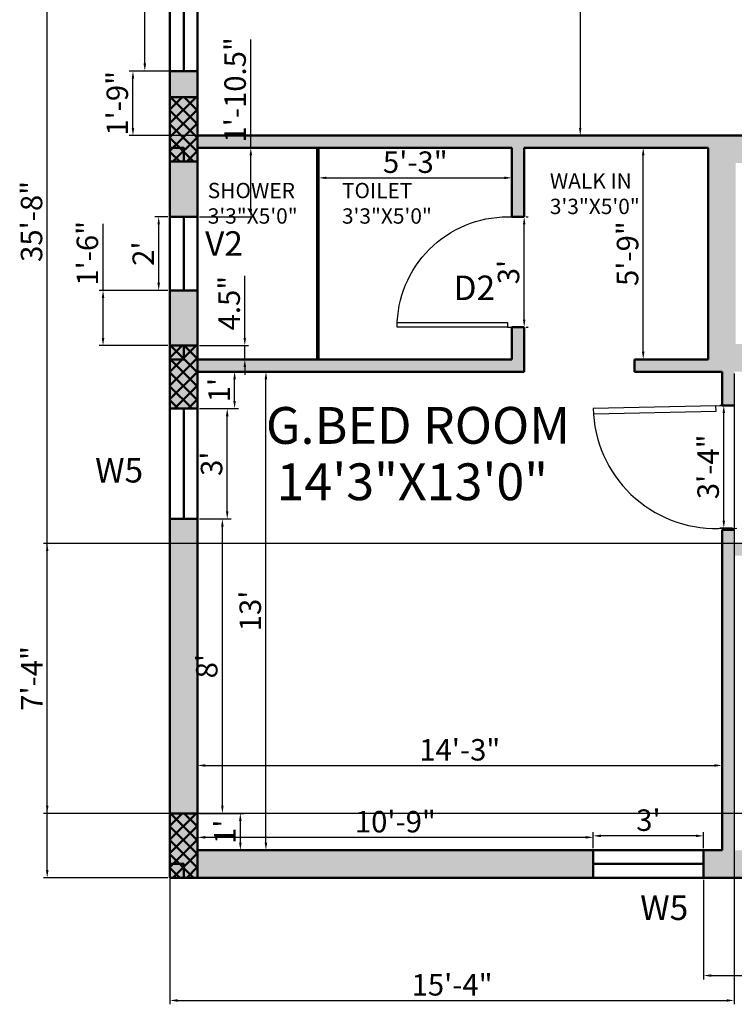
# Model space of a CAD drawing. Units: inches. Extents: x 1749 to 3550, y 1117 to 2383.
# Tile 1 of 15: x 1811 to 2044, y 1169 to 1490. Entities that reach past the tile are written whole.
import ezdxf

# ---------------------------------------------------------------- set-up
doc = ezdxf.new("R2010")
doc.units = ezdxf.units.IN
for name, color, linetype, lineweight in [('A-ANNO-DIMS', 2, 'Continuous', 18), ('A-ANNO-TEXT', 3, 'Continuous', 18), ('A-AREA-IDEN', 7, 'Continuous', 18), ('A-COLS', 10, 'Continuous', 50), ('A-DOOR', 30, 'Continuous', 25), ('A-WALL', 7, 'Continuous', 50), ('A-WALL-PATT', 8, 'Continuous', 13)]:
    doc.layers.add(name, color=color, linetype=linetype, lineweight=lineweight)
doc.styles.get("Standard").update_dxf_attribs({"font": 'arial.ttf'})
doc.dimstyles.new('ISO-25', dxfattribs={"dimtxt": 7, "dimasz": 2.5, "dimexe": 1.25, "dimexo": 0.625, "dimtad": 1, "dimdec": 1, "dimlunit": 3, "dimtxsty": 'Standard', "dimcen": 2.5, "dimadec": 0, "dimazin": 0, "dimtfac": 1, "dimtdec": 1, "dimtmove": 0, "dimatfit": 3, "dimfxl": 1, "dimarcsym": 0})

# ---------------------------------------------------------------- blocks, each defined once
blk = doc.blocks.new('*U12')
for p, q in [((0, 0), (0, 6)), ((40, 0), (40, 6))]:
    blk.add_line(p, q)
blk.add_lwpolyline([(0, 0), (0, -40), (1.75, -40), (1.75, 0)], close=True)
blk.add_arc((0, 0), 40, 270, 0)
blk = doc.blocks.new('*D16')
at = {"layer": 'A-ANNO-DIMS', "color": 0, "lineweight": -2, "ltscale": 0.5, "transparency": 16777216}
for p, q in [((1995.57, 1629.24), (1992.13, 1629.24)), ((1993.38, 1626.74), (1993.38, 1454.74)), ((1995.57, 1452.24), (1992.13, 1452.24))]:
    blk.add_line(p, q, dxfattribs=at)
at = {"layer": 'A-ANNO-DIMS', "color": 0, "ltscale": 0.5, "transparency": 16777216}
for points in [[(1992.96, 1626.74), (1993.8, 1626.74), (1993.38, 1629.24)], [(1992.96, 1454.74), (1993.8, 1454.74), (1993.38, 1452.24)]]:
    blk.add_solid(points, dxfattribs=at)
at = {"layer": 'Defpoints', "color": 0, "ltscale": 0.5, "transparency": 16777216}
for p in [(1996.2, 1629.24), (1993.38, 1452.24), (1996.2, 1452.24)]:
    blk.add_point(p, dxfattribs=at)
at = {"layer": 'A-ANNO-DIMS', "color": 0, "ltscale": 0.5, "transparency": 16777216, "insert": (1989.18, 1540.74), "char_height": 7, "attachment_point": 5, "rotation": 90}
blk.add_mtext('14\'-9"', dxfattribs=at)
blk = doc.blocks.new('*D21')
at = {"layer": 'A-ANNO-DIMS', "color": 0, "lineweight": -2, "ltscale": 0.5, "transparency": 16777216}
for p, q in [((2011.73, 1448.24), (2015.16, 1448.24)), ((2013.91, 1381.74), (2013.91, 1445.74)), ((2011.73, 1379.24), (2015.16, 1379.24))]:
    blk.add_line(p, q, dxfattribs=at)
at = {"layer": 'A-ANNO-DIMS', "color": 0, "ltscale": 0.5, "transparency": 16777216}
for points in [[(2013.49, 1445.74), (2014.33, 1445.74), (2013.91, 1448.24)], [(2013.49, 1381.74), (2014.33, 1381.74), (2013.91, 1379.24)]]:
    blk.add_solid(points, dxfattribs=at)
at = {"layer": 'Defpoints', "color": 0, "ltscale": 0.5, "transparency": 16777216}
for p in [(2011.1, 1448.24), (2013.91, 1448.24), (2011.1, 1379.24)]:
    blk.add_point(p, dxfattribs=at)
at = {"layer": 'A-ANNO-DIMS', "color": 0, "ltscale": 0.5, "transparency": 16777216, "insert": (2009.71, 1413.74), "char_height": 7, "attachment_point": 5, "rotation": 90}
blk.add_mtext('5\'-9"', dxfattribs=at)
blk = doc.blocks.new('*D22')
at = {"layer": 'A-ANNO-DIMS', "color": 0, "lineweight": -2, "ltscale": 0.5, "transparency": 16777216}
for p, q in [((1908.1, 1447.62), (1908.1, 1437.19)), ((1971.1, 1447.62), (1971.1, 1437.19)), ((1910.6, 1438.44), (1968.6, 1438.44))]:
    blk.add_line(p, q, dxfattribs=at)
at = {"layer": 'A-ANNO-DIMS', "color": 0, "ltscale": 0.5, "transparency": 16777216}
for points in [[(1910.6, 1438.86), (1910.6, 1438.03), (1908.1, 1438.44)], [(1968.6, 1438.86), (1968.6, 1438.03), (1971.1, 1438.44)]]:
    blk.add_solid(points, dxfattribs=at)
at = {"layer": 'Defpoints', "color": 0, "ltscale": 0.5, "transparency": 16777216}
for p in [(1908.1, 1448.24), (1971.1, 1448.24), (1971.1, 1438.44)]:
    blk.add_point(p, dxfattribs=at)
at = {"layer": 'A-ANNO-DIMS', "color": 0, "ltscale": 0.5, "transparency": 16777216, "insert": (1939.6, 1442.65), "char_height": 7, "attachment_point": 5}
blk.add_mtext('5\'-3"', dxfattribs=at)
blk = doc.blocks.new('*D23')
at = {"layer": 'A-ANNO-DIMS', "color": 0, "lineweight": -2, "ltscale": 0.5, "transparency": 16777216}
for p, q in [((1869.23, 1375.24), (1892.16, 1375.24)), ((1890.91, 1221.74), (1890.91, 1372.74)), ((1869.23, 1219.24), (1892.16, 1219.24))]:
    blk.add_line(p, q, dxfattribs=at)
at = {"layer": 'A-ANNO-DIMS', "color": 0, "ltscale": 0.5, "transparency": 16777216}
for points in [[(1890.49, 1372.74), (1891.33, 1372.74), (1890.91, 1375.24)], [(1890.49, 1221.74), (1891.33, 1221.74), (1890.91, 1219.24)]]:
    blk.add_solid(points, dxfattribs=at)
at = {"layer": 'Defpoints', "color": 0, "ltscale": 0.5, "transparency": 16777216}
for p in [(1868.6, 1375.24), (1890.91, 1375.24), (1868.6, 1219.24)]:
    blk.add_point(p, dxfattribs=at)
at = {"layer": 'A-ANNO-DIMS', "color": 0, "ltscale": 0.5, "transparency": 16777216, "insert": (1886.71, 1297.24), "char_height": 7, "attachment_point": 5, "rotation": 90}
blk.add_mtext("13'", dxfattribs=at)
blk = doc.blocks.new('*D24')
at = {"layer": 'A-ANNO-DIMS', "color": 0, "lineweight": -2, "ltscale": 0.5, "transparency": 16777216}
for p, q in [((1868.6, 1219.87), (1868.6, 1248.11)), ((1871.1, 1246.86), (2037.1, 1246.86)), ((2039.6, 1219.87), (2039.6, 1248.11))]:
    blk.add_line(p, q, dxfattribs=at)
at = {"layer": 'A-ANNO-DIMS', "color": 0, "ltscale": 0.5, "transparency": 16777216}
for points in [[(1871.1, 1247.28), (1871.1, 1246.44), (1868.6, 1246.86)], [(2037.1, 1247.28), (2037.1, 1246.44), (2039.6, 1246.86)]]:
    blk.add_solid(points, dxfattribs=at)
at = {"layer": 'Defpoints', "color": 0, "ltscale": 0.5, "transparency": 16777216}
for p in [(2039.6, 1246.86), (1868.6, 1219.24), (2039.6, 1219.24)]:
    blk.add_point(p, dxfattribs=at)
at = {"layer": 'A-ANNO-DIMS', "color": 0, "ltscale": 0.5, "transparency": 16777216, "insert": (1954.1, 1251.06), "char_height": 7, "attachment_point": 5}
blk.add_mtext('14\'-3"', dxfattribs=at)
blk = doc.blocks.new('*D61')
at = {"layer": 'A-ANNO-DIMS', "color": 0, "lineweight": -2, "ltscale": 0.5, "transparency": 16777216}
for p, q in [((2033.6, 1209.62), (2033.6, 1177.12)), ((2057.1, 1209.62), (2057.1, 1177.12)), ((2036.1, 1178.37), (2054.6, 1178.37)), ((2057.1, 1178.37), (2092.4, 1178.37))]:
    blk.add_line(p, q, dxfattribs=at)
at = {"layer": 'A-ANNO-DIMS', "color": 0, "ltscale": 0.5, "transparency": 16777216}
for points in [[(2036.1, 1178.79), (2036.1, 1177.95), (2033.6, 1178.37)], [(2054.6, 1178.79), (2054.6, 1177.95), (2057.1, 1178.37)]]:
    blk.add_solid(points, dxfattribs=at)
at = {"layer": 'Defpoints', "color": 0, "ltscale": 0.5, "transparency": 16777216}
for p in [(2033.6, 1210.24), (2057.1, 1210.24), (2057.1, 1178.37)]:
    blk.add_point(p, dxfattribs=at)
at = {"layer": 'A-ANNO-DIMS', "color": 0, "ltscale": 0.5, "transparency": 16777216, "insert": (2076, 1182.57), "char_height": 7, "attachment_point": 5}
blk.add_mtext('1\'-11.5"', dxfattribs=at)
blk = doc.blocks.new('*D62')
at = {"layer": 'A-ANNO-DIMS', "color": 0, "lineweight": -2, "ltscale": 0.5, "transparency": 16777216}
for p, q in [((1997.6, 1219.87), (1997.6, 1225.16)), ((2031.1, 1223.91), (2000.1, 1223.91)), ((2033.6, 1219.87), (2033.6, 1225.16))]:
    blk.add_line(p, q, dxfattribs=at)
at = {"layer": 'A-ANNO-DIMS', "color": 0, "ltscale": 0.5, "transparency": 16777216}
for points in [[(2000.1, 1224.33), (2000.1, 1223.5), (1997.6, 1223.91)], [(2031.1, 1224.33), (2031.1, 1223.5), (2033.6, 1223.91)]]:
    blk.add_solid(points, dxfattribs=at)
at = {"layer": 'Defpoints', "color": 0, "ltscale": 0.5, "transparency": 16777216}
for p in [(1997.6, 1223.91), (1997.6, 1219.24), (2033.6, 1219.24)]:
    blk.add_point(p, dxfattribs=at)
at = {"layer": 'A-ANNO-DIMS', "color": 0, "ltscale": 0.5, "transparency": 16777216, "insert": (2015.6, 1228.12), "char_height": 7, "attachment_point": 5}
blk.add_mtext("3'", dxfattribs=at)
blk = doc.blocks.new('*D63')
at = {"layer": 'A-ANNO-DIMS', "color": 0, "lineweight": -2, "ltscale": 0.5, "transparency": 16777216}
for p, q in [((1868.6, 1219.87), (1868.6, 1224.68)), ((1995.1, 1223.43), (1871.1, 1223.43)), ((1997.6, 1219.87), (1997.6, 1224.68))]:
    blk.add_line(p, q, dxfattribs=at)
at = {"layer": 'A-ANNO-DIMS', "color": 0, "ltscale": 0.5, "transparency": 16777216}
for points in [[(1871.1, 1223.85), (1871.1, 1223.01), (1868.6, 1223.43)], [(1995.1, 1223.85), (1995.1, 1223.01), (1997.6, 1223.43)]]:
    blk.add_solid(points, dxfattribs=at)
at = {"layer": 'Defpoints', "color": 0, "ltscale": 0.5, "transparency": 16777216}
for p in [(1868.6, 1223.43), (1868.6, 1219.24), (1997.6, 1219.24)]:
    blk.add_point(p, dxfattribs=at)
at = {"layer": 'A-ANNO-DIMS', "color": 0, "ltscale": 0.5, "transparency": 16777216, "insert": (1933.1, 1227.63), "char_height": 7, "attachment_point": 5}
blk.add_mtext('10\'-9"', dxfattribs=at)
blk = doc.blocks.new('*D64')
at = {"layer": 'A-ANNO-DIMS', "color": 0, "lineweight": -2, "ltscale": 0.5, "transparency": 16777216}
for p, q in [((1869.23, 1231.24), (1883.82, 1231.24)), ((1882.57, 1221.74), (1882.57, 1228.74)), ((1869.23, 1219.24), (1883.82, 1219.24))]:
    blk.add_line(p, q, dxfattribs=at)
at = {"layer": 'A-ANNO-DIMS', "color": 0, "ltscale": 0.5, "transparency": 16777216}
for points in [[(1882.15, 1228.74), (1882.99, 1228.74), (1882.57, 1231.24)], [(1882.15, 1221.74), (1882.99, 1221.74), (1882.57, 1219.24)]]:
    blk.add_solid(points, dxfattribs=at)
at = {"layer": 'Defpoints', "color": 0, "ltscale": 0.5, "transparency": 16777216}
for p in [(1868.6, 1231.24), (1882.57, 1231.24), (1868.6, 1219.24)]:
    blk.add_point(p, dxfattribs=at)
at = {"layer": 'A-ANNO-DIMS', "color": 0, "ltscale": 0.5, "transparency": 16777216, "insert": (1878.43, 1225.24), "char_height": 7, "attachment_point": 5, "rotation": 90}
blk.add_mtext("1'", dxfattribs=at)
blk = doc.blocks.new('*D65')
at = {"layer": 'A-ANNO-DIMS', "color": 0, "lineweight": -2, "ltscale": 0.5, "transparency": 16777216}
for p, q in [((1869.23, 1327.24), (1877.97, 1327.24)), ((1876.72, 1233.74), (1876.72, 1324.74)), ((1869.23, 1231.24), (1877.97, 1231.24))]:
    blk.add_line(p, q, dxfattribs=at)
at = {"layer": 'A-ANNO-DIMS', "color": 0, "ltscale": 0.5, "transparency": 16777216}
for points in [[(1876.3, 1324.74), (1877.13, 1324.74), (1876.72, 1327.24)], [(1876.3, 1233.74), (1877.13, 1233.74), (1876.72, 1231.24)]]:
    blk.add_solid(points, dxfattribs=at)
at = {"layer": 'Defpoints', "color": 0, "ltscale": 0.5, "transparency": 16777216}
for p in [(1868.6, 1327.24), (1876.72, 1327.24), (1868.6, 1231.24)]:
    blk.add_point(p, dxfattribs=at)
at = {"layer": 'A-ANNO-DIMS', "color": 0, "ltscale": 0.5, "transparency": 16777216, "insert": (1872.52, 1279.24), "char_height": 7, "attachment_point": 5, "rotation": 90}
blk.add_mtext("8'", dxfattribs=at)
blk = doc.blocks.new('*D66')
at = {"layer": 'A-ANNO-DIMS', "color": 0, "lineweight": -2, "ltscale": 0.5, "transparency": 16777216}
for p, q in [((1869.23, 1363.24), (1879.54, 1363.24)), ((1878.29, 1329.74), (1878.29, 1360.74)), ((1869.23, 1327.24), (1879.54, 1327.24))]:
    blk.add_line(p, q, dxfattribs=at)
at = {"layer": 'A-ANNO-DIMS', "color": 0, "ltscale": 0.5, "transparency": 16777216}
for points in [[(1877.87, 1360.74), (1878.71, 1360.74), (1878.29, 1363.24)], [(1877.87, 1329.74), (1878.71, 1329.74), (1878.29, 1327.24)]]:
    blk.add_solid(points, dxfattribs=at)
at = {"layer": 'Defpoints', "color": 0, "ltscale": 0.5, "transparency": 16777216}
for p in [(1868.6, 1363.24), (1878.29, 1363.24), (1868.6, 1327.24)]:
    blk.add_point(p, dxfattribs=at)
at = {"layer": 'A-ANNO-DIMS', "color": 0, "ltscale": 0.5, "transparency": 16777216, "insert": (1874.09, 1345.24), "char_height": 7, "attachment_point": 5, "rotation": 90}
blk.add_mtext("3'", dxfattribs=at)
blk = doc.blocks.new('*D67')
at = {"layer": 'A-ANNO-DIMS', "color": 0, "lineweight": -2, "ltscale": 0.5, "transparency": 16777216}
for p, q in [((1869.23, 1375.24), (1881.95, 1375.24)), ((1880.7, 1365.74), (1880.7, 1372.74)), ((1869.23, 1363.24), (1881.95, 1363.24))]:
    blk.add_line(p, q, dxfattribs=at)
at = {"layer": 'A-ANNO-DIMS', "color": 0, "ltscale": 0.5, "transparency": 16777216}
for points in [[(1880.28, 1372.74), (1881.11, 1372.74), (1880.7, 1375.24)], [(1880.28, 1365.74), (1881.11, 1365.74), (1880.7, 1363.24)]]:
    blk.add_solid(points, dxfattribs=at)
at = {"layer": 'Defpoints', "color": 0, "ltscale": 0.5, "transparency": 16777216}
for p in [(1868.6, 1375.24), (1880.7, 1375.24), (1868.6, 1363.24)]:
    blk.add_point(p, dxfattribs=at)
at = {"layer": 'A-ANNO-DIMS', "color": 0, "ltscale": 0.5, "transparency": 16777216, "insert": (1876.56, 1369.24), "char_height": 7, "attachment_point": 5, "rotation": 90}
blk.add_mtext("1'", dxfattribs=at)
blk = doc.blocks.new('*D68')
at = {"layer": 'A-ANNO-DIMS', "color": 0, "lineweight": -2, "ltscale": 0.5, "transparency": 16777216}
for p, q in [((1884.02, 1386.24), (1884.02, 1406.48)), ((1869.23, 1383.74), (1885.27, 1383.74)), ((1884.02, 1379.24), (1884.02, 1383.74)), ((1869.23, 1379.24), (1885.27, 1379.24)), ((1884.02, 1376.74), (1884.02, 1374.24))]:
    blk.add_line(p, q, dxfattribs=at)
at = {"layer": 'A-ANNO-DIMS', "color": 0, "ltscale": 0.5, "transparency": 16777216}
for points in [[(1883.6, 1386.24), (1884.43, 1386.24), (1884.02, 1383.74)], [(1883.6, 1376.74), (1884.43, 1376.74), (1884.02, 1379.24)]]:
    blk.add_solid(points, dxfattribs=at)
at = {"layer": 'Defpoints', "color": 0, "ltscale": 0.5, "transparency": 16777216}
for p in [(1868.6, 1383.74), (1884.02, 1383.74), (1868.6, 1379.24)]:
    blk.add_point(p, dxfattribs=at)
at = {"layer": 'A-ANNO-DIMS', "color": 0, "ltscale": 0.5, "transparency": 16777216, "insert": (1879.83, 1397.61), "char_height": 7, "attachment_point": 5, "rotation": 90}
blk.add_mtext('4.5"', dxfattribs=at)
blk = doc.blocks.new('*D69')
at = {"layer": 'A-ANNO-DIMS', "color": 0, "lineweight": -2, "ltscale": 0.5, "transparency": 16777216}
for p, q in [((1837.81, 1401.74), (1837.81, 1423.44)), ((1858.98, 1401.74), (1836.56, 1401.74)), ((1837.81, 1386.24), (1837.81, 1399.24)), ((1858.98, 1383.74), (1836.56, 1383.74))]:
    blk.add_line(p, q, dxfattribs=at)
at = {"layer": 'A-ANNO-DIMS', "color": 0, "ltscale": 0.5, "transparency": 16777216}
for points in [[(1837.39, 1399.24), (1838.23, 1399.24), (1837.81, 1401.74)], [(1837.39, 1386.24), (1838.23, 1386.24), (1837.81, 1383.74)]]:
    blk.add_solid(points, dxfattribs=at)
at = {"layer": 'Defpoints', "color": 0, "ltscale": 0.5, "transparency": 16777216}
for p in [(1837.81, 1401.74), (1859.6, 1401.74), (1859.6, 1383.74)]:
    blk.add_point(p, dxfattribs=at)
at = {"layer": 'A-ANNO-DIMS', "color": 0, "ltscale": 0.5, "transparency": 16777216, "insert": (1833.61, 1413.84), "char_height": 7, "attachment_point": 5, "rotation": 90}
blk.add_mtext('1\'-6"', dxfattribs=at)
blk = doc.blocks.new('*D70')
at = {"layer": 'A-ANNO-DIMS', "color": 0, "lineweight": -2, "ltscale": 0.5, "transparency": 16777216}
for p, q in [((1858.98, 1425.74), (1854.7, 1425.74)), ((1855.95, 1404.24), (1855.95, 1423.24)), ((1858.98, 1401.74), (1854.7, 1401.74))]:
    blk.add_line(p, q, dxfattribs=at)
at = {"layer": 'A-ANNO-DIMS', "color": 0, "ltscale": 0.5, "transparency": 16777216}
for points in [[(1855.53, 1423.24), (1856.36, 1423.24), (1855.95, 1425.74)], [(1855.53, 1404.24), (1856.36, 1404.24), (1855.95, 1401.74)]]:
    blk.add_solid(points, dxfattribs=at)
at = {"layer": 'Defpoints', "color": 0, "ltscale": 0.5, "transparency": 16777216}
for p in [(1855.95, 1425.74), (1859.6, 1425.74), (1859.6, 1401.74)]:
    blk.add_point(p, dxfattribs=at)
at = {"layer": 'A-ANNO-DIMS', "color": 0, "ltscale": 0.5, "transparency": 16777216, "insert": (1851.81, 1413.74), "char_height": 7, "attachment_point": 5, "rotation": 90}
blk.add_mtext("2'", dxfattribs=at)
blk = doc.blocks.new('*D71')
at = {"layer": 'A-ANNO-DIMS', "color": 0, "lineweight": -2, "ltscale": 0.5, "transparency": 16777216}
for p, q in [((1885.97, 1448.24), (1885.97, 1483.54)), ((1869.23, 1448.24), (1887.22, 1448.24)), ((1885.97, 1428.24), (1885.97, 1445.74)), ((1869.23, 1425.74), (1887.22, 1425.74))]:
    blk.add_line(p, q, dxfattribs=at)
at = {"layer": 'A-ANNO-DIMS', "color": 0, "ltscale": 0.5, "transparency": 16777216}
for points in [[(1885.56, 1445.74), (1886.39, 1445.74), (1885.97, 1448.24)], [(1885.56, 1428.24), (1886.39, 1428.24), (1885.97, 1425.74)]]:
    blk.add_solid(points, dxfattribs=at)
at = {"layer": 'Defpoints', "color": 0, "ltscale": 0.5, "transparency": 16777216}
for p in [(1868.6, 1448.24), (1885.97, 1448.24), (1868.6, 1425.74)]:
    blk.add_point(p, dxfattribs=at)
at = {"layer": 'A-ANNO-DIMS', "color": 0, "ltscale": 0.5, "transparency": 16777216, "insert": (1881.77, 1467.14), "char_height": 7, "attachment_point": 5, "rotation": 90}
blk.add_mtext('1\'-10.5"', dxfattribs=at)
blk = doc.blocks.new('*D72')
at = {"layer": 'A-ANNO-DIMS', "color": 0, "lineweight": -2, "ltscale": 0.5, "transparency": 16777216}
for p, q in [((1867.98, 1473.24), (1846.31, 1473.24)), ((1847.56, 1454.74), (1847.56, 1470.74)), ((1867.98, 1452.24), (1846.31, 1452.24))]:
    blk.add_line(p, q, dxfattribs=at)
at = {"layer": 'A-ANNO-DIMS', "color": 0, "ltscale": 0.5, "transparency": 16777216}
for points in [[(1847.14, 1470.74), (1847.97, 1470.74), (1847.56, 1473.24)], [(1847.14, 1454.74), (1847.97, 1454.74), (1847.56, 1452.24)]]:
    blk.add_solid(points, dxfattribs=at)
at = {"layer": 'Defpoints', "color": 0, "ltscale": 0.5, "transparency": 16777216}
for p in [(1847.56, 1473.24), (1868.6, 1473.24), (1868.6, 1452.24)]:
    blk.add_point(p, dxfattribs=at)
at = {"layer": 'A-ANNO-DIMS', "color": 0, "ltscale": 0.5, "transparency": 16777216, "insert": (1843.36, 1462.74), "char_height": 7, "attachment_point": 5, "rotation": 90}
blk.add_mtext('1\'-9"', dxfattribs=at)
blk = doc.blocks.new('*D73')
at = {"layer": 'A-ANNO-DIMS', "color": 0, "lineweight": -2, "ltscale": 0.5, "transparency": 16777216}
for p, q in [((1858.98, 1593.24), (1850.18, 1593.24)), ((1851.43, 1475.74), (1851.43, 1590.74)), ((1858.98, 1473.24), (1850.18, 1473.24))]:
    blk.add_line(p, q, dxfattribs=at)
at = {"layer": 'A-ANNO-DIMS', "color": 0, "ltscale": 0.5, "transparency": 16777216}
for points in [[(1851.01, 1590.74), (1851.84, 1590.74), (1851.43, 1593.24)], [(1851.01, 1475.74), (1851.84, 1475.74), (1851.43, 1473.24)]]:
    blk.add_solid(points, dxfattribs=at)
at = {"layer": 'Defpoints', "color": 0, "ltscale": 0.5, "transparency": 16777216}
for p in [(1851.43, 1593.24), (1859.6, 1593.24), (1859.6, 1473.24)]:
    blk.add_point(p, dxfattribs=at)
at = {"layer": 'A-ANNO-DIMS', "color": 0, "ltscale": 0.5, "transparency": 16777216, "insert": (1847.23, 1533.24), "char_height": 7, "attachment_point": 5, "rotation": 90}
blk.add_mtext("10'", dxfattribs=at)
blk = doc.blocks.new('*D96')
at = {"layer": 'A-ANNO-DIMS', "color": 0, "lineweight": -2, "ltscale": 0.5, "transparency": 16777216}
for p, q in [((1975.73, 1425.74), (1976.35, 1425.74)), ((1975.1, 1392.24), (1975.1, 1423.24)), ((1975.73, 1389.74), (1976.35, 1389.74))]:
    blk.add_line(p, q, dxfattribs=at)
at = {"layer": 'A-ANNO-DIMS', "color": 0, "ltscale": 0.5, "transparency": 16777216}
for points in [[(1974.69, 1423.24), (1975.52, 1423.24), (1975.1, 1425.74)], [(1974.69, 1392.24), (1975.52, 1392.24), (1975.1, 1389.74)]]:
    blk.add_solid(points, dxfattribs=at)
at = {"layer": 'Defpoints', "color": 0, "ltscale": 0.5, "transparency": 16777216}
for p in [(1975.1, 1425.74), (1975.1, 1425.74), (1975.1, 1389.74)]:
    blk.add_point(p, dxfattribs=at)
at = {"layer": 'A-ANNO-DIMS', "color": 0, "ltscale": 0.5, "transparency": 16777216, "insert": (1970.9, 1407.74), "char_height": 7, "attachment_point": 5, "rotation": 90}
blk.add_mtext("3'", dxfattribs=at)
blk = doc.blocks.new('*D97')
at = {"layer": 'A-ANNO-DIMS', "color": 0, "lineweight": -2, "ltscale": 0.5, "transparency": 16777216}
for p, q in [((2042.16, 1364.23), (2038.93, 1364.23)), ((2040.18, 1326.73), (2040.18, 1361.73)), ((2042.98, 1324.23), (2038.93, 1324.23))]:
    blk.add_line(p, q, dxfattribs=at)
at = {"layer": 'A-ANNO-DIMS', "color": 0, "ltscale": 0.5, "transparency": 16777216}
for points in [[(2039.77, 1361.73), (2040.6, 1361.73), (2040.18, 1364.23)], [(2039.77, 1326.73), (2040.6, 1326.73), (2040.18, 1324.23)]]:
    blk.add_solid(points, dxfattribs=at)
at = {"layer": 'Defpoints', "color": 0, "ltscale": 0.5, "transparency": 16777216}
for p in [(2040.18, 1364.23), (2042.78, 1364.23), (2043.6, 1324.23)]:
    blk.add_point(p, dxfattribs=at)
at = {"layer": 'A-ANNO-DIMS', "color": 0, "ltscale": 0.5, "transparency": 16777216, "insert": (2035.98, 1344.23), "char_height": 7, "attachment_point": 5, "rotation": 90}
blk.add_mtext('3\'-4"', dxfattribs=at)
blk = doc.blocks.new('*D173')
at = {"layer": 'A-ANNO-DIMS', "color": 0, "lineweight": -2, "ltscale": 0.5, "transparency": 16777216}
for p, q in [((1858.98, 1638.24), (1818.35, 1638.24)), ((1819.6, 1212.74), (1819.6, 1635.74)), ((1858.98, 1210.24), (1818.35, 1210.24))]:
    blk.add_line(p, q, dxfattribs=at)
at = {"layer": 'A-ANNO-DIMS', "color": 0, "ltscale": 0.5, "transparency": 16777216}
for points in [[(1819.19, 1635.74), (1820.02, 1635.74), (1819.6, 1638.24)], [(1819.19, 1212.74), (1820.02, 1212.74), (1819.6, 1210.24)]]:
    blk.add_solid(points, dxfattribs=at)
at = {"layer": 'Defpoints', "color": 0, "ltscale": 0.5, "transparency": 16777216}
for p in [(1819.6, 1638.24), (1859.6, 1638.24), (1859.6, 1210.24)]:
    blk.add_point(p, dxfattribs=at)
at = {"layer": 'A-ANNO-DIMS', "color": 0, "ltscale": 0.5, "transparency": 16777216, "insert": (1815.4, 1424.24), "char_height": 7, "attachment_point": 5, "rotation": 90}
blk.add_mtext('35\'-8"', dxfattribs=at)
blk = doc.blocks.new('*D176')
at = {"layer": 'A-ANNO-DIMS', "color": 0, "lineweight": -2, "ltscale": 0.5, "transparency": 16777216}
for p, q in [((2102.98, 1319.24), (1818.35, 1319.24)), ((1819.6, 1233.74), (1819.6, 1316.74)), ((2102.98, 1231.24), (1818.35, 1231.24))]:
    blk.add_line(p, q, dxfattribs=at)
at = {"layer": 'A-ANNO-DIMS', "color": 0, "ltscale": 0.5, "transparency": 16777216}
for points in [[(1819.19, 1316.74), (1820.02, 1316.74), (1819.6, 1319.24)], [(1819.19, 1233.74), (1820.02, 1233.74), (1819.6, 1231.24)]]:
    blk.add_solid(points, dxfattribs=at)
at = {"layer": 'Defpoints', "color": 0, "ltscale": 0.5, "transparency": 16777216}
for p in [(1819.6, 1319.24), (2103.6, 1319.24), (2103.6, 1231.24)]:
    blk.add_point(p, dxfattribs=at)
at = {"layer": 'A-ANNO-DIMS', "color": 0, "ltscale": 0.5, "transparency": 16777216, "insert": (1815.48, 1275.24), "char_height": 7, "attachment_point": 5, "rotation": 90}
blk.add_mtext('7\'-4"', dxfattribs=at)
blk = doc.blocks.new('*D178')
at = {"layer": 'A-ANNO-DIMS', "color": 0, "lineweight": -2, "ltscale": 0.5, "transparency": 16777216}
for p, q in [((1859.6, 1378.62), (1859.6, 1168.99)), ((2043.6, 1374.62), (2043.6, 1168.99)), ((1862.1, 1170.24), (2041.1, 1170.24))]:
    blk.add_line(p, q, dxfattribs=at)
at = {"layer": 'A-ANNO-DIMS', "color": 0, "ltscale": 0.5, "transparency": 16777216}
for points in [[(1862.1, 1170.66), (1862.1, 1169.83), (1859.6, 1170.24)], [(2041.1, 1170.66), (2041.1, 1169.83), (2043.6, 1170.24)]]:
    blk.add_solid(points, dxfattribs=at)
at = {"layer": 'Defpoints', "color": 0, "ltscale": 0.5, "transparency": 16777216}
for p in [(1859.6, 1379.24), (2043.6, 1375.24), (2043.6, 1170.24)]:
    blk.add_point(p, dxfattribs=at)
at = {"layer": 'A-ANNO-DIMS', "color": 0, "ltscale": 0.5, "transparency": 16777216, "insert": (1951.6, 1174.44), "char_height": 7, "attachment_point": 5}
blk.add_mtext('15\'-4"', dxfattribs=at)

msp = doc.modelspace()

# ---------------------------------------------------------------- hatches: boundary and pattern name
at = {"layer": 'A-COLS', "ltscale": 10}
h = msp.add_hatch(dxfattribs=at)
h.set_pattern_fill('ANSI37', color=256, angle=90)
h.set_pattern_definition([(135, (3226.7103, -207.5015), (-2.245064, -2.245064), []), (225, (3226.7103, -207.5015), (2.245064, -2.245064), [])])
h.paths.add_polyline_path([(1868.6, 1464.74), (1859.6, 1464.74), (1859.6, 1443.74), (1868.6, 1443.74)])
h = msp.add_hatch(color=256, dxfattribs=at)
h.dxf.hatch_style = 1
h.paths.add_polyline_path([(1859.6, 1448.24), (1859.6, 1443.74), (1864.1, 1443.74), (1864.1, 1448.24)])
h = msp.add_hatch(color=256, dxfattribs=at)
h.dxf.hatch_style = 1
h.paths.add_polyline_path([(1859.6, 1383.74), (1859.6, 1379.24), (1864.1, 1379.24), (1864.1, 1383.74)])
h = msp.add_hatch(dxfattribs=at)
h.set_pattern_fill('ANSI37', color=256, angle=90)
h.set_pattern_definition([(135, (3226.7103, -288.5015), (-2.245064, -2.245064), []), (225, (3226.7103, -288.5015), (2.245064, -2.245064), [])])
h.paths.add_polyline_path([(1868.6, 1383.74), (1859.6, 1383.74), (1859.6, 1363.24), (1868.6, 1363.24)])
h = msp.add_hatch(dxfattribs=at)
h.set_pattern_fill('ANSI37', color=256, angle=90)
h.set_pattern_definition([(135, (3226.7103, -441.0015), (-2.245064, -2.245064), []), (225, (3226.7103, -441.0015), (2.245064, -2.245064), [])])
h.paths.add_polyline_path([(1868.6, 1231.24), (1859.6, 1231.24), (1859.6, 1210.24), (1868.6, 1210.24)])
h = msp.add_hatch(color=256, dxfattribs=at)
h.dxf.hatch_style = 1
h.paths.add_polyline_path([(1859.6, 1214.74), (1859.6, 1210.24), (1864.1, 1210.24), (1864.1, 1214.74)])
at = {"layer": 'A-WALL-PATT', "ltscale": 10}
h = msp.add_hatch(color=256, dxfattribs=at)
h.dxf.hatch_style = 1
h.paths.add_polyline_path([(1971.1, 1448.24), (1971.1, 1425.74), (1975.1, 1425.74), (1975.1, 1448.24), (2035.1, 1448.24), (2035.1, 1379.24), (2011.1, 1379.24), (2011.1, 1375.24), (2039.6, 1375.24), (2039.6, 1364.24), (2043.6, 1364.24), (2043.6, 1375.24), (2113.1, 1375.24), (2113.1, 1392.24), (2104.1, 1392.24), (2104.1, 1379.24), (2044.1, 1379.24), (2044.1, 1443.24), (2104.1, 1443.24), (2104.1, 1434.24), (2113.1, 1434.24), (2113.1, 1452.24), (2104.1, 1452.24), (1868.6, 1452.24), (1868.6, 1473.24), (1859.6, 1473.24), (1859.6, 1425.74), (1868.6, 1425.74), (1868.6, 1448.24), (1907.6, 1448.24), (1908.1, 1448.24)])
h = msp.add_hatch(color=256, dxfattribs=at)
h.dxf.hatch_style = 1
h.paths.add_polyline_path([(2044.1, 1384.24), (2044.1, 1443.24), (2104.1, 1443.24), (2104.1, 1434.24), (2113.1, 1434.24), (2113.1, 1447.74), (2108.6, 1447.74), (2108.6, 1452.24), (2104.1, 1452.24), (1868.6, 1452.24), (1868.6, 1448.24), (1907.6, 1448.24), (1908.1, 1448.24), (1971.1, 1448.24), (1971.1, 1425.74), (1975.1, 1425.74), (1975.1, 1448.24), (2035.1, 1448.24), (2035.1, 1379.24), (2011.1, 1379.24), (2011.1, 1375.24), (2039.6, 1375.24), (2039.6, 1364.24), (2043.6, 1364.24), (2043.6, 1375.24), (2092.1, 1375.24), (2092.1, 1384.24)])
h.paths.add_polyline_path([(2092.1, 1384.24), (2092.1, 1375.24), (2108.6, 1375.24), (2108.6, 1379.74), (2113.1, 1379.74), (2113.1, 1384.24)], flags=17)
h = msp.add_hatch(color=256, dxfattribs=at)
h.dxf.hatch_style = 1
h.paths.add_polyline_path([(1975.1, 1375.24), (1975.1, 1379.24), (1975.1, 1389.74), (1971.1, 1389.74), (1971.1, 1379.24), (1908.1, 1379.24), (1907.6, 1379.24), (1868.6, 1379.24), (1868.6, 1401.74), (1859.6, 1401.74), (1859.6, 1363.24), (1868.6, 1363.24), (1868.6, 1375.24)])
h = msp.add_hatch(color=256, dxfattribs=at)
h.dxf.hatch_style = 1
h.paths.add_polyline_path([(1997.6, 1210.24), (1997.6, 1219.24), (1868.6, 1219.24), (1868.6, 1327.24), (1859.6, 1327.24), (1859.6, 1210.24)])
h = msp.add_hatch(color=256, dxfattribs=at)
h.dxf.hatch_style = 1
h.paths.add_polyline_path([(2039.6, 1219.24), (2033.6, 1219.24), (2033.6, 1210.24), (2057.1, 1210.24), (2057.1, 1219.24), (2043.6, 1219.24), (2043.6, 1315.24), (2058.6, 1315.24), (2058.6, 1319.24), (2043.6, 1319.24), (2043.6, 1323.74), (2039.6, 1323.74)])

# ---------------------------------------------------------------- linework, layer by layer
at = {"layer": 'A-COLS', "ltscale": 10}
for points in [[(1859.6, 1443.74), (1859.6, 1464.74), (1868.6, 1464.74), (1868.6, 1443.74)], [(1859.6, 1448.24), (1864.1, 1448.24), (1864.1, 1443.74), (1859.6, 1443.74)], [(1859.6, 1383.74), (1864.1, 1383.74), (1864.1, 1379.24), (1859.6, 1379.24)], [(1859.6, 1363.24), (1859.6, 1383.74), (1868.6, 1383.74), (1868.6, 1363.24)], [(1859.6, 1210.24), (1859.6, 1231.24), (1868.6, 1231.24), (1868.6, 1210.24)], [(1859.6, 1214.74), (1864.1, 1214.74), (1864.1, 1210.24), (1859.6, 1210.24)]]:
    msp.add_lwpolyline(points, close=True, dxfattribs=at)
at = {"layer": 'A-WALL', "ltscale": 0.2}
for p, q in [((1859.6, 1638.24), (1859.6, 1210.24)), ((1868.6, 1629.24), (1868.6, 1452.24)), ((1864.1, 1593.24), (1864.1, 1473.24)), ((1868.6, 1473.24), (1859.6, 1473.24)), ((1868.6, 1452.24), (2104.1, 1452.24)), ((1868.6, 1448.24), (1907.6, 1448.24)), ((1868.6, 1448.24), (1868.6, 1379.24)), ((1907.6, 1448.24), (1907.6, 1379.24)), ((1907.83, 1379.24), (1907.83, 1448.24)), ((1908.1, 1448.24), (1908.1, 1379.24)), ((1908.1, 1448.24), (1971.1, 1448.24)), ((1971.1, 1448.24), (1971.1, 1425.74)), ((1975.1, 1448.24), (1975.1, 1425.74)), ((1975.1, 1448.24), (2035.1, 1448.24)), ((2035.1, 1448.24), (2035.1, 1379.24)), ((1868.6, 1425.74), (1859.6, 1425.74)), ((1864.1, 1401.74), (1864.1, 1425.74)), ((1971.1, 1425.74), (1975.1, 1425.74)), ((1868.6, 1401.74), (1859.6, 1401.74)), ((1971.1, 1389.74), (1975.1, 1389.74)), ((1971.1, 1389.74), (1971.1, 1379.24)), ((1975.1, 1389.74), (1975.1, 1379.24)), ((1868.6, 1379.24), (1907.6, 1379.24)), ((1908.1, 1379.24), (1971.1, 1379.24)), ((1975.1, 1379.24), (1975.1, 1375.24)), ((2011.1, 1379.24), (2035.1, 1379.24)), ((2011.1, 1379.24), (2011.1, 1375.24)), ((1868.6, 1375.24), (1975.1, 1375.24)), ((1868.6, 1375.24), (1868.6, 1219.24)), ((2011.1, 1375.24), (2039.6, 1375.24)), ((2039.6, 1375.24), (2039.6, 1364.24)), ((1868.6, 1363.24), (1859.6, 1363.24)), ((1864.1, 1327.24), (1864.1, 1363.24)), ((2043.6, 1364.24), (2039.6, 1364.24)), ((1868.6, 1327.24), (1859.6, 1327.24)), ((2043.6, 1323.74), (2039.6, 1323.74)), ((2039.6, 1323.74), (2039.6, 1219.24)), ((1868.6, 1219.24), (2039.6, 1219.24)), ((1997.6, 1219.24), (1997.6, 1210.24)), ((2033.6, 1219.24), (2033.6, 1210.24)), ((1997.6, 1214.74), (2033.6, 1214.74)), ((1859.6, 1210.24), (2103.6, 1210.24))]:
    msp.add_line(p, q, dxfattribs=at)
at = {"layer": 'A-WALL', "ltscale": 10}
for p, q in [((1907.6, 1448.24), (1908.1, 1448.24)), ((1907.6, 1379.24), (1908.1, 1379.24))]:
    msp.add_line(p, q, dxfattribs=at)

# ---------------------------------------------------------------- block references
at = {"layer": 'A-DOOR', "xscale": -0.9, "yscale": 0.9, "zscale": 0.9, "rotation": 270}
msp.add_blockref('*U12', (1969.7, 1389.74), dxfattribs=at)
at = {"layer": 'A-DOOR', "rotation": 271.1803398379497}
msp.add_blockref('*U12', (2037.61, 1364.12), dxfattribs=at)

# ---------------------------------------------------------------- texts
at = {"layer": 'A-ANNO-TEXT', "ltscale": 0.5}
for s, p in [('V2', (1871.07, 1413.04)), ('D2', (1952.07, 1398.59)), ('W5', (1835.23, 1339.12)), ('W5', (2012.94, 1196.49))]:
    msp.add_text(s, height=8, dxfattribs=at).set_placement(p)
at = {"layer": 'A-AREA-IDEN', "ltscale": 0.5}
for s, height, p in [('WALK IN', 5, (1983.47, 1434.94)), ('SHOWER', 5, (1871.94, 1431.81)), ('TOILET', 5, (1915.69, 1431.81)), ('3\'3"X5\'0"', 5, (1983.47, 1426.64)), ('3\'3"X5\'0"', 5, (1871.94, 1423.51)), ('3\'3"X5\'0"', 5, (1915.69, 1423.51)), ('14\'3"X13\'0"', 12, (1894.37, 1333.36))]:
    msp.add_text(s, height=height, dxfattribs=at).set_placement(p)
msp.add_text('G.BED ROOM', height=12, rotation=0.0333, dxfattribs=at).set_placement((1890.91, 1351.71))

# ---------------------------------------------------------------- dimensions: what is measured, and where the dimension line sits
at = {"layer": 'A-ANNO-DIMS', "ltscale": 0.5}
for base, p1, p2, override, picture, middle in [((1819.6, 1638.24), (1859.6, 1210.24), (1859.6, 1638.24), {"dimdec": 1, "dimlfac": 1, "dimrnd": 0, "dimzin": 1, "dimdsep": 46, "dimlunit": 4, "dimfrac": 2}, '*D173', (1815.4, 1424.24)), ((1993.38, 1452.24), (1996.2, 1629.24), (1996.2, 1452.24), {"dimclrd": 0, "dimclre": 0, "dimclrt": 0}, '*D16', (1989.18, 1540.74)), ((1851.43, 1593.24), (1859.6, 1473.24), (1859.6, 1593.24), {"dimclrd": 0, "dimclre": 0, "dimclrt": 0}, '*D73', (1847.23, 1533.24)), ((1885.97, 1448.24), (1868.6, 1425.74), (1868.6, 1448.24), {"dimclrd": 0, "dimclre": 0, "dimclrt": 0}, '*D71', (1881.77, 1467.14)), ((1847.56, 1473.24), (1868.6, 1452.24), (1868.6, 1473.24), {"dimclrd": 0, "dimclre": 0, "dimclrt": 0}, '*D72', (1843.36, 1462.74)), ((2013.91, 1448.24), (2011.1, 1379.24), (2011.1, 1448.24), {"dimclrd": 0, "dimclre": 0, "dimclrt": 0}, '*D21', (2009.71, 1413.74)), ((1855.95, 1425.74), (1859.6, 1401.74), (1859.6, 1425.74), {"dimclrd": 0, "dimclre": 0, "dimclrt": 0}, '*D70', (1851.81, 1413.74)), ((1975.1, 1425.74), (1975.1, 1389.74), (1975.1, 1425.74), {"dimclrd": 0, "dimclre": 0, "dimclrt": 0}, '*D96', (1970.9, 1407.74)), ((1837.81, 1401.74), (1859.6, 1383.74), (1859.6, 1401.74), {"dimclrd": 0, "dimclre": 0, "dimclrt": 0}, '*D69', (1833.61, 1413.84)), ((1884.02, 1383.74), (1868.6, 1379.24), (1868.6, 1383.74), {"dimclrd": 0, "dimclre": 0, "dimclrt": 0}, '*D68', (1879.83, 1397.61)), ((1890.91, 1375.24), (1868.6, 1219.24), (1868.6, 1375.24), {"dimclrd": 0, "dimclre": 0, "dimclrt": 0}, '*D23', (1886.71, 1297.24)), ((1880.7, 1375.24), (1868.6, 1363.24), (1868.6, 1375.24), {"dimclrd": 0, "dimclre": 0, "dimclrt": 0}, '*D67', (1876.56, 1369.24)), ((1878.29, 1363.24), (1868.6, 1327.24), (1868.6, 1363.24), {"dimclrd": 0, "dimclre": 0, "dimclrt": 0}, '*D66', (1874.09, 1345.24)), ((2040.18, 1364.23), (2043.6, 1324.23), (2042.78, 1364.23), {"dimclrd": 0, "dimclre": 0, "dimclrt": 0}, '*D97', (2035.98, 1344.23)), ((1876.72, 1327.24), (1868.6, 1231.24), (1868.6, 1327.24), {"dimclrd": 0, "dimclre": 0, "dimclrt": 0}, '*D65', (1872.52, 1279.24)), ((1819.6, 1319.24), (2103.6, 1231.24), (2103.6, 1319.24), {"dimdec": 1, "dimlfac": 1, "dimrnd": 0, "dimzin": 1, "dimdsep": 46, "dimlunit": 4, "dimfrac": 2}, '*D176', (1815.48, 1275.24)), ((1882.57, 1231.24), (1868.6, 1219.24), (1868.6, 1231.24), {"dimclrd": 0, "dimclre": 0, "dimclrt": 0}, '*D64', (1878.43, 1225.24))]:
    dim = msp.add_linear_dim(base=base, p1=p1, p2=p2, angle=90, dimstyle='ISO-25', override=override, dxfattribs=at)
    dim.commit()
    dim.dimension.update_dxf_attribs({"geometry": picture, "text_midpoint": middle})
for base, p1, p2, override, picture, middle in [((1971.1, 1438.44), (1908.1, 1448.24), (1971.1, 1448.24), {"dimclrd": 0, "dimclre": 0, "dimclrt": 0}, '*D22', (1939.6, 1442.65)), ((2043.6, 1170.24), (1859.6, 1379.24), (2043.6, 1375.24), {"dimdec": 1, "dimlfac": 1, "dimrnd": 0, "dimzin": 1, "dimdsep": 46, "dimlunit": 4, "dimfrac": 2}, '*D178', (1951.6, 1174.44)), ((2039.6, 1246.86), (1868.6, 1219.24), (2039.6, 1219.24), {"dimclrd": 0, "dimclre": 0, "dimclrt": 0}, '*D24', (1954.1, 1251.06)), ((1997.6, 1223.91), (2033.6, 1219.24), (1997.6, 1219.24), {"dimclrd": 0, "dimclre": 0, "dimclrt": 0}, '*D62', (2015.6, 1228.12)), ((1868.6, 1223.43), (1997.6, 1219.24), (1868.6, 1219.24), {"dimclrd": 0, "dimclre": 0, "dimclrt": 0}, '*D63', (1933.1, 1227.63)), ((2057.1, 1178.37), (2033.6, 1210.24), (2057.1, 1210.24), {"dimclrd": 0, "dimclre": 0, "dimclrt": 0}, '*D61', (2076, 1182.57))]:
    dim = msp.add_linear_dim(base=base, p1=p1, p2=p2, dimstyle='ISO-25', override=override, dxfattribs=at)
    dim.commit()
    dim.dimension.update_dxf_attribs({"geometry": picture, "text_midpoint": middle})

doc.saveas('drawing.dxf')
